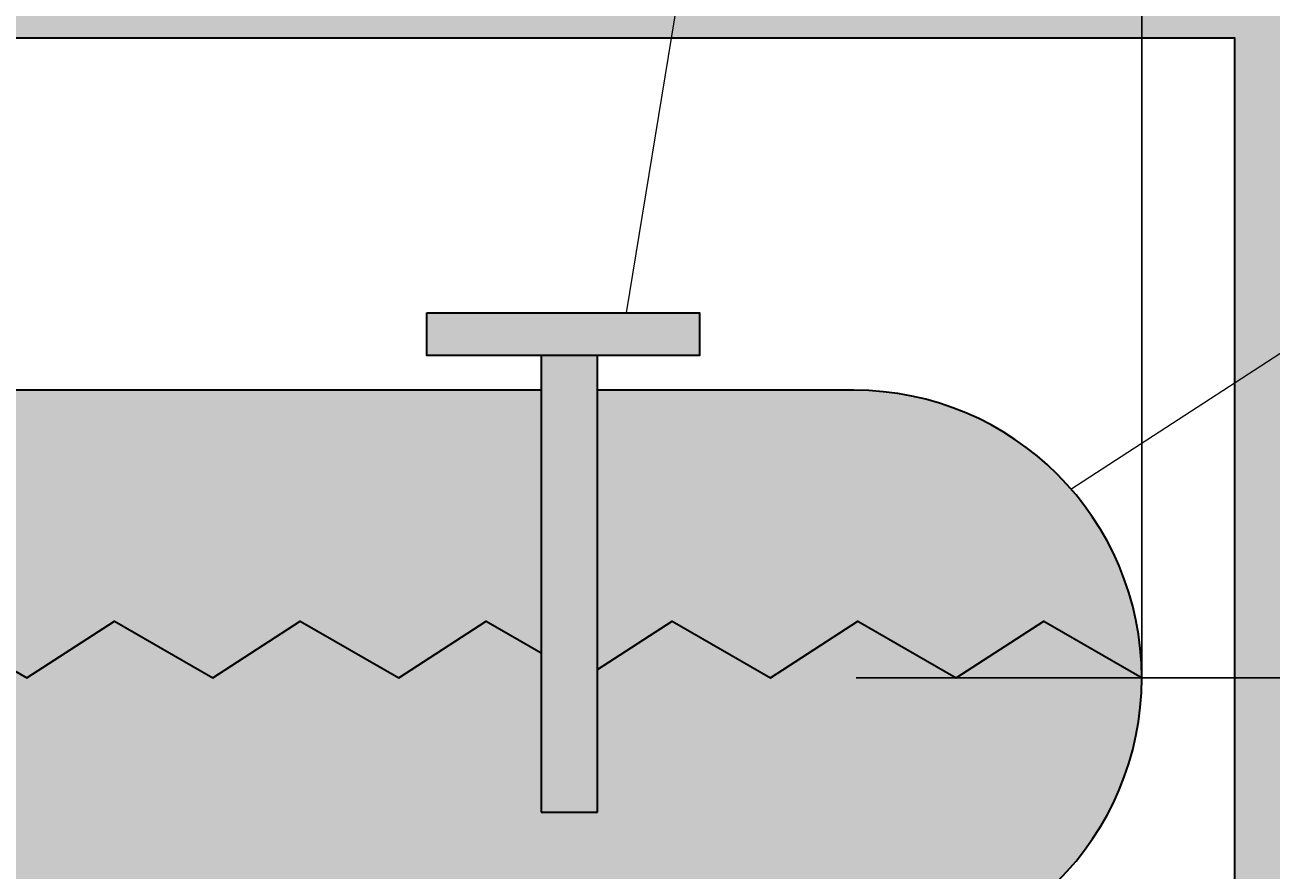
# Model space of a CAD drawing. Units: inches. Extents: x -1 to 292, y -3 to 199.
# Tile 30 of 52: x 146 to 181, y 95 to 118. Entities that reach past the tile are written whole.
import ezdxf

# ---------------------------------------------------------------- set-up
doc = ezdxf.new("R2010")
doc.units = ezdxf.units.IN
doc.header["$MEASUREMENT"] = 0
for name, color, linetype, lineweight in [('M-ANNO-LEAD', 2, 'Continuous', 18), ('M-DIMS', 2, 'Continuous', 18), ('M-EQPM', 7, 'Continuous', 35), ('M-PATT', 8, 'Continuous', 13)]:
    doc.layers.add(name, color=color, linetype=linetype, lineweight=lineweight)
doc.styles.get("Standard").update_dxf_attribs({"font": 'arial.ttf'})
doc.dimstyles.get("Standard").update_dxf_attribs({"dimtxt": 0.18, "dimasz": 0.18, "dimexe": 0.18, "dimexo": 0.0625, "dimgap": 0.09, "dimtad": 0, "dimtih": 1, "dimtoh": 1, "dimdec": 4, "dimzin": 0, "dimdsep": 46, "dimtxsty": 'Standard', "dimcen": 0.09, "dimadec": 0, "dimazin": 0, "dimtfac": 1, "dimtdec": 4, "dimtofl": 0, "dimtmove": 0, "dimatfit": 3, "dimfxl": 1, "dimtolj": 1, "dimtzin": 0, "dimarcsym": 0})

# ---------------------------------------------------------------- blocks, each defined once
blk = doc.blocks.new('*D9')
at = {"layer": 'Defpoints', "color": 0, "transparency": 16777216}
for p in [(177.053, 174.363), (49.924, 99.774), (177.053, 99.774)]:
    blk.add_point(p, dxfattribs=at)
at = {"layer": 'M-DIMS', "color": 0, "lineweight": -2, "transparency": 16777216}
for p, q in [((49.924, 99.836), (49.924, 174.543)), ((50.104, 174.363), (113.033, 174.363)), ((176.873, 174.363), (113.943, 174.363)), ((177.053, 99.836), (177.053, 174.543))]:
    blk.add_line(p, q, dxfattribs=at)
at = {"layer": 'M-DIMS', "color": 0, "transparency": 16777216}
for points in [[(50.104, 174.393), (50.104, 174.333), (49.924, 174.363)], [(176.873, 174.393), (176.873, 174.333), (177.053, 174.363)]]:
    blk.add_solid(points, dxfattribs=at)
at = {"layer": 'M-DIMS', "color": 0, "transparency": 16777216, "insert": (113.488, 174.363), "char_height": 0.18, "attachment_point": 5}
blk.add_mtext('\\A1;127.13', dxfattribs=at)
blk = doc.blocks.new('*D10')
at = {"layer": 'Defpoints', "color": 0, "transparency": 16777216}
for p in [(169.176, 99.774), (169.176, 43.391), (292.04, 43.391)]:
    blk.add_point(p, dxfattribs=at)
at = {"layer": 'M-DIMS', "color": 0, "lineweight": -2, "transparency": 16777216}
for p, q in [((169.239, 99.774), (292.22, 99.774)), ((292.04, 99.594), (292.04, 71.764)), ((292.04, 43.571), (292.04, 71.4)), ((169.239, 43.391), (292.22, 43.391))]:
    blk.add_line(p, q, dxfattribs=at)
at = {"layer": 'M-DIMS', "color": 0, "transparency": 16777216}
for points in [[(292.01, 99.594), (292.07, 99.594), (292.04, 99.774)], [(292.01, 43.571), (292.07, 43.571), (292.04, 43.391)]]:
    blk.add_solid(points, dxfattribs=at)
at = {"layer": 'M-DIMS', "color": 0, "transparency": 16777216, "insert": (292.04, 71.582), "char_height": 0.18, "attachment_point": 5}
blk.add_mtext('\\A1;56.38', dxfattribs=at)

msp = doc.modelspace()

# ---------------------------------------------------------------- hatches: boundary and pattern name
at = {"layer": 'M-PATT'}
h = msp.add_hatch(color=256, dxfattribs=at)
h.set_gradient(color1=(0, 127, 0), color2=(0, 127, 0), tint=1, name='CYLINDER')
h.paths.add_polyline_path([(164.5186, 119.2985), (129.9293, 119.2985), (129.9293, 117.2985), (164.1897, 117.2985)])
h.paths.add_polyline_path([(181.5897, 119.2985), (164.5186, 119.2985), (164.1897, 117.2985), (179.5897, 117.2985), (179.5897, 107.8518), (181.5897, 109.1506)])
h.paths.add_polyline_path([(181.5897, 109.1506), (179.5897, 107.8518), (179.5897, 36.2698), (198.4159, 36.2698), (198.4159, 38.2698), (181.5897, 38.2698)])
h.paths.add_polyline_path([(115.4883, 126.765), (111.4883, 126.765), (111.4883, 114.6589), (115.4883, 114.6589)])
h.paths.add_polyline_path([(123.408, 119.2985), (115.4883, 119.2985), (115.4883, 117.2985), (123.408, 117.2985)])
h.paths.add_polyline_path([(115.4883, 112.6589), (111.4883, 112.6589), (111.4883, 106.9941), (115.4883, 106.9941)])
h.paths.add_polyline_path([(120.9032, 106.9941), (106.0735, 106.9941), (106.0735, 105.9941), (120.9032, 105.9941)])
h.paths.add_polyline_path([(236.4209, 117.5104), (234.9209, 117.5104), (234.9209, 97.1861), (236.4209, 97.1861)])
h.paths.add_polyline_path([(236.4209, 126.4904), (234.9209, 126.4904), (234.9209, 118.9331), (236.4209, 118.9331)])
h.paths.add_polyline_path([(244.9552, 125.7269), (242.9552, 125.7269), (242.9552, 116.8562), (244.9552, 116.8562)])
h.paths.add_polyline_path([(244.9552, 115.1721), (242.9552, 115.1721), (242.9552, 109.7385), (244.9552, 109.7385)])
h.paths.add_polyline_path([(248.4468, 109.7385), (239.4637, 109.7385), (239.4637, 109.4289), (248.4468, 109.4289)])
h = msp.add_hatch(color=256, dxfattribs=at)
h.set_gradient(color1=(0, 127, 0), color2=(0, 127, 0), tint=1, name='CYLINDER')
h.paths.add_polyline_path([(160.6222, 96.1027), (162.1623, 96.1027), (162.1623, 108.5995), (160.6222, 108.5995)])
h.paths.add_polyline_path([(157.4899, 108.5995), (164.9536, 108.5995), (164.9536, 109.7655), (157.4899, 109.7655)])
h = msp.add_hatch(color=256, dxfattribs=at)
h.set_gradient(color1=(237, 31, 36), color2=(242, 113, 114), tint=1, name='CYLINDER')
h.paths.add_polyline_path([(106.0735, 105.9941), (106.0735, 106.9941), (108.0603, 106.9941), (107.8488, 107.6501), (57.8007, 107.6501, 0.4142136), (49.9241, 99.7735), (52.3176, 101.3278), (55.0097, 99.7735), (57.4032, 101.3278), (60.0953, 99.7735), (62.4888, 101.3278), (65.1809, 99.7735), (67.5744, 101.3278), (70.2665, 99.7735), (72.66, 101.3278), (75.3521, 99.7735), (77.7456, 101.3278), (80.4377, 99.7735), (82.8312, 101.3278), (85.5233, 99.7735), (87.9168, 101.3278), (90.6089, 99.7735), (93.0024, 101.3278), (95.6945, 99.7735), (98.088, 101.3278), (100.7801, 99.7735), (103.1736, 101.3278), (105.8657, 99.7735), (108.2592, 101.3278), (110.9513, 99.7735), (113.3448, 101.3278), (116.0369, 99.7735), (118.4304, 101.3278), (121.1225, 99.7735), (123.516, 101.3278), (126.2082, 99.7735), (128.6016, 101.3278), (131.2938, 99.7735), (133.6872, 101.3278), (136.3794, 99.7735), (138.7728, 101.3278), (141.465, 99.7735), (143.8584, 101.3278), (146.5506, 99.7735), (148.944, 101.3278), (151.6362, 99.7735), (154.0296, 101.3278), (156.7218, 99.7735), (159.1152, 101.3278), (160.6222, 100.4578), (160.6222, 107.6501), (115.4883, 107.6501), (115.4883, 106.9941), (120.9032, 106.9941), (120.9032, 105.9941), (120.9032, 103.3981), (106.0735, 103.3981)])
h.paths.add_polyline_path([(169.176, 107.6501), (162.1623, 107.6501), (162.1623, 100.004), (164.2008, 101.3278), (166.893, 99.7735), (169.2864, 101.3278), (171.9786, 99.7735), (174.372, 101.3278), (177.0526, 99.7802, 0.4139642)])
h.paths.add_polyline_path([(111.4883, 107.6501), (107.8488, 107.6501), (108.0603, 106.9941), (111.4883, 106.9941)], flags=17)
h.paths.add_polyline_path([(61.6788, 91.897), (57.8007, 91.897, -0.1099266), (54.4604, 92.6403), (43.2011, 92.6403), (23.9502, 84.4688), (23.9502, 58.376), (43.2011, 47.2615), (50.9409, 47.2615, -0.2705926), (57.8007, 51.2672), (61.6788, 51.2672)])
h.paths.add_polyline_path([(73.6788, 91.897), (70.6788, 91.897), (70.6788, 51.2672), (73.6788, 51.2672)])
h.paths.add_polyline_path([(79.6788, 91.897), (76.6788, 91.897), (76.6788, 51.2672), (79.6788, 51.2672)])
h.paths.add_polyline_path([(67.6788, 91.897), (64.6788, 91.897), (64.6788, 51.2672), (67.6788, 51.2672)])
h.paths.add_polyline_path([(101.6788, 91.897), (82.6788, 91.897), (82.6788, 51.2672), (101.6788, 51.2672)])
h.paths.add_polyline_path([(107.6788, 91.897), (104.6788, 91.897), (104.6788, 51.2672), (107.6788, 51.2672)])
h.paths.add_polyline_path([(113.6788, 91.897), (110.6788, 91.897), (110.6788, 51.2672), (113.6788, 51.2672)])
h.paths.add_polyline_path([(119.6788, 91.897), (116.6788, 91.897), (116.6788, 51.2672), (119.6788, 51.2672)])
h.paths.add_polyline_path([(141.6788, 91.897), (122.6788, 91.897), (122.6788, 51.2672), (141.6788, 51.2672)])
h.paths.add_polyline_path([(147.6788, 91.897), (144.6788, 91.897), (144.6788, 51.2672), (147.6788, 51.2672)])
h.paths.add_polyline_path([(153.6788, 91.897), (150.6788, 91.897), (150.6788, 51.2672), (153.6788, 51.2672)])
h.paths.add_polyline_path([(159.6788, 91.897), (156.6788, 91.897), (156.6788, 51.2672), (159.6788, 51.2672)])
h.paths.add_polyline_path([(179.5897, 92.6403), (172.5163, 92.6403, -0.1099266), (169.176, 91.897), (162.6788, 91.897), (162.6788, 51.2672), (169.176, 51.2672, -0.2705926), (176.0358, 47.2615), (179.5897, 47.2615)])
h.paths.add_polyline_path([(203.0265, 84.4688), (183.7755, 92.6403), (181.5897, 92.6403), (181.5897, 47.2615), (183.7755, 47.2615), (203.0265, 58.376)])
h.paths.add_polyline_path([(184.4188, 61.52), (200.7224, 61.52), (200.7224, 77.7532), (184.4188, 77.7532)], flags=24)
h = msp.add_hatch(color=256, dxfattribs=at)
h.set_gradient(color1=(0, 255, 255), color2=(0, 255, 255), tint=1)
h.paths.add_polyline_path([(75.3521, 99.7735), (72.66, 101.3278), (70.2665, 99.7735), (67.5744, 101.3278), (65.1809, 99.7735), (62.4888, 101.3278), (60.0953, 99.7735), (57.4032, 101.3278), (55.0097, 99.7735), (52.3176, 101.3278), (49.9241, 99.7735, 0.4142136), (57.8007, 91.897), (61.6788, 91.897), (61.6788, 51.2672), (57.8007, 51.2672, 0.8088808), (54.5813, 36.2021), (65.0947, 51.2672), (64.6788, 51.2672), (64.6788, 91.897), (67.6788, 91.897), (67.6788, 51.2672), (65.0947, 51.2672), (54.5813, 36.2021, 0.1056561), (57.8007, 35.5141), (169.176, 35.5141, 1), (169.176, 51.2672), (162.6788, 51.2672), (162.6788, 91.897), (169.176, 91.897, 0.4144629), (177.0526, 99.7802), (174.372, 101.3278), (171.9786, 99.7735), (169.2864, 101.3278), (166.893, 99.7735), (164.2008, 101.3278), (162.1623, 100.004), (162.1623, 96.1027), (160.6222, 96.1027), (160.6222, 100.4578), (159.1152, 101.3278), (156.7218, 99.7735), (154.0296, 101.3278), (151.6362, 99.7735), (148.944, 101.3278), (146.5506, 99.7735), (143.8584, 101.3278), (141.465, 99.7735), (138.7728, 101.3278), (136.3794, 99.7735), (133.6872, 101.3278), (131.2938, 99.7735), (128.6016, 101.3278), (126.2082, 99.7735), (123.516, 101.3278), (121.1225, 99.7735), (118.4304, 101.3278), (116.0369, 99.7735), (113.3448, 101.3278), (110.9513, 99.7735), (108.2592, 101.3278), (105.8657, 99.7735), (103.1736, 101.3278), (100.7801, 99.7735), (98.088, 101.3278), (95.6945, 99.7735), (93.0024, 101.3278), (90.6089, 99.7735), (87.9168, 101.3278), (85.5233, 99.7735), (82.8312, 101.3278), (80.4377, 99.7735), (77.7456, 101.3278)])
h.paths.add_polyline_path([(79.6788, 91.897), (79.6788, 51.2672), (76.6788, 51.2672), (76.6788, 91.897)], flags=16)
h.paths.add_polyline_path([(73.6788, 91.897), (73.6788, 51.2672), (70.6788, 51.2672), (70.6788, 91.897)], flags=16)
h.paths.add_polyline_path([(82.6788, 91.897), (101.6788, 91.897), (101.6788, 51.2672), (82.6788, 51.2672)], flags=16)
h.paths.add_polyline_path([(104.6788, 91.897), (107.6788, 91.897), (107.6788, 51.2672), (104.6788, 51.2672)], flags=16)
h.paths.add_polyline_path([(110.6788, 91.897), (113.6788, 91.897), (113.6788, 51.2672), (110.6788, 51.2672)], flags=16)
h.paths.add_polyline_path([(116.6788, 91.897), (119.6788, 91.897), (119.6788, 51.2672), (116.6788, 51.2672)], flags=16)
h.paths.add_polyline_path([(122.6788, 91.897), (141.6788, 91.897), (141.6788, 51.2672), (144.6788, 51.2672), (144.6788, 91.897), (147.6788, 91.897), (147.6788, 51.2672), (122.6788, 51.2672)], flags=16)
h.paths.add_polyline_path([(150.6788, 91.897), (153.6788, 91.897), (153.6788, 51.2672), (150.6788, 51.2672)], flags=16)
h.paths.add_polyline_path([(156.6788, 91.897), (159.6788, 91.897), (159.6788, 51.2672), (156.6788, 51.2672)], flags=16)

# ---------------------------------------------------------------- linework, layer by layer
at = {"layer": 'M-ANNO-LEAD'}
for p, q in [((162.951, 109.7655), (166.6813, 132.451)), ((175.1158, 104.9464), (184.6596, 111.1442))]:
    msp.add_line(p, q, dxfattribs=at)
at = {"layer": 'M-EQPM'}
for p, q in [((160.6222, 108.5995), (160.6222, 96.1027)), ((162.1623, 96.1027), (162.1623, 108.5995)), ((160.6222, 96.1027), (162.1623, 96.1027))]:
    msp.add_line(p, q, dxfattribs=at)
for points in [[(129.9293, 117.2985), (179.5897, 117.2985), (179.5897, 36.2698)], [(160.6222, 107.6501), (115.4883, 107.6501)], [(141.465, 99.7735), (143.8584, 101.3278), (146.5506, 99.7735)], [(146.5506, 99.7735), (148.944, 101.3278), (151.6362, 99.7735)], [(151.6362, 99.7735), (154.0296, 101.3278), (156.7218, 99.7735)], [(156.7218, 99.7735), (159.1152, 101.3278), (160.6222, 100.4578)], [(162.1623, 100.004), (164.2008, 101.3278), (166.893, 99.7735)], [(166.893, 99.7735), (169.2864, 101.3278), (171.9786, 99.7735)], [(171.9786, 99.7735), (174.372, 101.3278), (177.0642, 99.7735)]]:
    msp.add_lwpolyline(points, dxfattribs=at)
msp.add_lwpolyline([(157.4899, 109.7655), (164.9536, 109.7655), (164.9536, 108.5995), (157.4899, 108.5995)], close=True, dxfattribs=at)
msp.add_lwpolyline([(162.6788, 91.897), (169.176, 91.897, 1), (169.176, 107.6501), (162.1623, 107.6501)], format="xyb", dxfattribs=at)

# ---------------------------------------------------------------- dimensions: what is measured, and where the dimension line sits
at = {"layer": 'M-DIMS'}
dim = msp.add_linear_dim(base=(177.0526, 174.3627), p1=(49.9241, 99.7735), p2=(177.0526, 99.7735), dimstyle='Standard', override={"dimdec": 2, "dimlfac": 1, "dimrnd": 0, "dimzin": 0, "dimdsep": 46, "dimlunit": 2}, dxfattribs=at)
dim.commit()
dim.dimension.update_dxf_attribs({"geometry": '*D9', "text_midpoint": (113.4883, 174.3627)})
dim = msp.add_linear_dim(base=(292.0399, 43.3906), p1=(169.176, 99.7735), p2=(169.176, 43.3906), angle=90, dimstyle='Standard', override={"dimdec": 2, "dimlfac": 1, "dimrnd": 0, "dimzin": 0, "dimdsep": 46, "dimlunit": 2}, dxfattribs=at)
dim.commit()
dim.dimension.update_dxf_attribs({"geometry": '*D10', "text_midpoint": (292.0399, 71.5821)})

doc.saveas('drawing.dxf')
